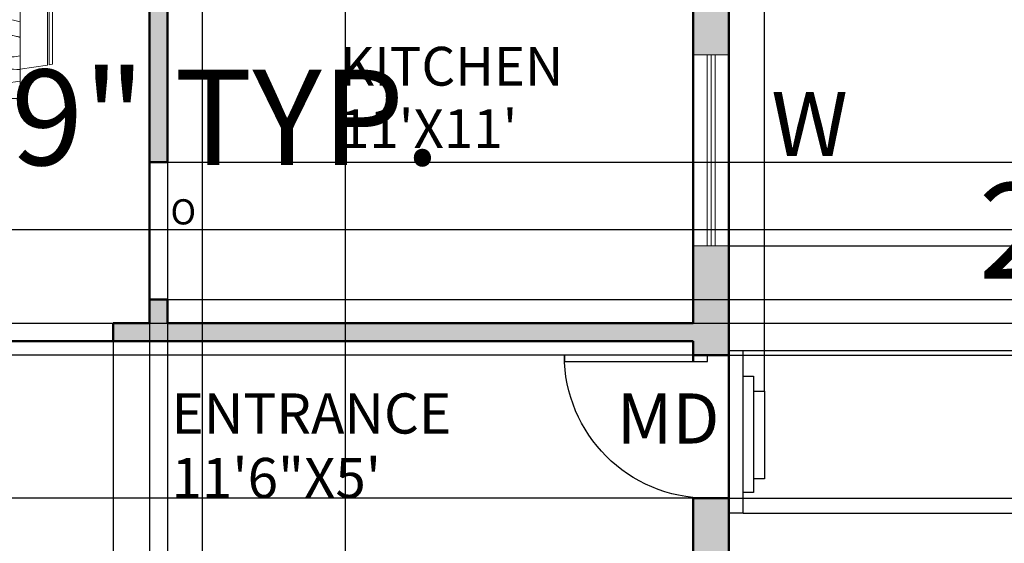
# Model space of a CAD drawing. Units: inches. Extents: x -166 to 1001, y 0 to 688.
# Tile 8 of 11: x 361 to 608, y 287 to 419. Entities that reach past the tile are written whole.
import ezdxf

# ---------------------------------------------------------------- set-up
doc = ezdxf.new("R2010")
doc.units = ezdxf.units.IN
doc.header["$MEASUREMENT"] = 0
for name, color, linetype, lineweight in [('A-ANNO-DIMS', 1, 'Continuous', 18), ('A-ANNO-TEXT', 2, 'Continuous', 25), ('A-AREA-IDEN', 2, 'Continuous', 25), ('A-DOOR', 6, 'Continuous', 25), ('A-FLOR-STRS', 7, 'Continuous', 25), ('A-GLAZ', 130, 'Continuous', 18), ('A-WALL-PATT', 5, 'Continuous', 13), ('FURNITURE', 11, 'Continuous', 18), ('WALLS', 250, 'Continuous', 50)]:
    doc.layers.add(name, color=color, linetype=linetype, lineweight=lineweight)
doc.styles.get("Standard").update_dxf_attribs({"font": 'arial.ttf'})
doc.dimstyles.get("Standard").update_dxf_attribs({"dimtxt": 24, "dimasz": 7, "dimexe": 0.18, "dimexo": 0.0625, "dimgap": 0.09, "dimtad": 0, "dimtih": 1, "dimtoh": 1, "dimdec": 0, "dimzin": 0, "dimdsep": 46, "dimlunit": 3, "dimtxsty": 'Standard', "dimcen": 0.09, "dimadec": 0, "dimazin": 0, "dimtfac": 1, "dimtdec": 0, "dimtofl": 0, "dimtmove": 0, "dimatfit": 3, "dimfxl": 1, "dimtolj": 1, "dimtzin": 0, "dimarcsym": 0})

# ---------------------------------------------------------------- blocks, each defined once
blk = doc.blocks.new('Dining Set - 36 x 72 in.')
for p, q in [((-22.2343, 26.00059), (-23.4847, 17.99762)), ((-22.2304, 26), (-5.7608, 26)), ((-22, 27.5), (-22.1562, 26.50042)), ((-5.8416, 26.5), (-22.1534, 26.5)), ((-22, 27.5), (-6, 27.5)), ((-5.8437, 26.49966), (-6, 27.5)), ((-4.5152, 17.99762), (-5.7655, 25.99926)), ((5.7657, 26.00059), (4.5153, 17.99762)), ((5.7696, 26), (22.2392, 26)), ((6, 27.5), (5.8438, 26.50042)), ((22.1584, 26.5), (5.8466, 26.5)), ((6, 27.5), (22, 27.5)), ((22.1563, 26.49966), (22, 27.5)), ((23.4848, 17.99762), (22.2345, 25.99926)), ((36, 18), (-36, 18)), ((-36, 18), (-36, -18)), ((36, -18), (36, 18)), ((-44.0006, 8.23428), (-35.9976, 9.48474)), ((44.0006, 8.23428), (35.9976, 9.48474)), ((-45.5, 8), (-44.5004, 8.15617)), ((-45.5, 8), (-45.5, -8)), ((-44.5, -8.15843), (-44.5, 8.15338)), ((-44, 8.23041), (-44, -8.23915)), ((44, 8.23041), (44, -8.23915)), ((44.5, -8.15843), (44.5, 8.15338)), ((45.5, 8), (44.5005, 8.15617)), ((45.5, 8), (45.5, -8)), ((-44.4997, -8.15631), (-45.5, -8)), ((-35.9976, -9.48476), (-43.9993, -8.2345)), ((35.9976, -9.48476), (43.9993, -8.2345)), ((44.4997, -8.15631), (45.5, -8)), ((-36, -18), (36, -18)), ((-22.2343, -26.0006), (-23.4847, -17.99762)), ((-4.5152, -17.99762), (-5.7655, -25.99928)), ((5.7657, -26.0006), (4.5153, -17.99762)), ((23.4848, -17.99762), (22.2345, -25.99928)), ((-22.2304, -26), (-5.7608, -26)), ((-22, -27.5), (-22.1562, -26.50044)), ((-5.8416, -26.5), (-22.1534, -26.5)), ((-22, -27.5), (-6, -27.5)), ((-5.8437, -26.49967), (-6, -27.5)), ((5.7696, -26), (22.2392, -26)), ((6, -27.5), (5.8438, -26.50044)), ((22.1584, -26.5), (5.8466, -26.5)), ((6, -27.5), (22, -27.5)), ((22.1563, -26.49967), (22, -27.5))]:
    blk.add_line(p, q)
for points in [[(-36, 15), (-31.1772, 14.97754), (-26.8079, 14.91406), (-22.8538, 14.81543), (-19.276, 14.6875), (-16.0362, 14.53613), (-13.0957, 14.36718), (-10.4159, 14.18652), (-7.9583, 14), (-5.6904, 13.81315), (-3.6035, 13.63021), (-1.6954, 13.45508), (0.0365, 13.29166), (1.5945, 13.14388), (2.9811, 13.01562), (4.1988, 12.9108), (5.25, 12.83333), (6.1393, 12.78613), (6.8802, 12.76823), (7.4883, 12.77767), (7.9792, 12.8125), (8.3685, 12.87077), (8.6719, 12.95052), (8.9049, 13.0498), (9.0833, 13.16666), (9.2205, 13.29899), (9.3216, 13.44401), (9.3895, 13.59879), (9.4271, 13.76041), (9.4373, 13.92594), (9.4232, 14.09245), (9.3875, 14.257), (9.3333, 14.41666), (9.2638, 14.56917), (9.1836, 14.71484), (9.0975, 14.85465), (9.0104, 14.98958), (8.9272, 15.1206), (8.8529, 15.2487), (8.7922, 15.37483), (8.75, 15.5), (8.7305, 15.62467), (8.7344, 15.74739), (8.7617, 15.86621), (8.8125, 15.97916), (8.8867, 16.08431), (8.9844, 16.17968), (9.1055, 16.26334), (9.25, 16.33333), (9.4189, 16.38802), (9.6172, 16.42708), (9.8506, 16.45052), (10.125, 16.45833), (10.4463, 16.45052), (10.8203, 16.42708), (11.2529, 16.38802), (11.75, 16.33333), (12.3184, 16.26318), (12.9694, 16.17838), (13.7151, 16.07991), (14.5677, 15.96875), (15.5395, 15.84586), (16.6426, 15.71224), (17.8893, 15.56884), (19.2917, 15.41666), (20.859, 15.25667), (22.5879, 15.08984), (24.4721, 14.91715), (26.5052, 14.73958), (28.6809, 14.5581), (30.9929, 14.3737), (33.4347, 14.18733), (36, 14)], [(-36, 10), (-28.9766, 10.14274), (-23.1725, 10.20442), (-18.4241, 10.19775), (-14.5677, 10.13541), (-11.4399, 10.03011), (-8.877, 9.89453), (-6.7154, 9.74137), (-4.7917, 9.58333), (-2.9698, 9.43082), (-1.2246, 9.28515), (0.4415, 9.14534), (2.026, 9.01041), (3.5266, 8.87939), (4.9408, 8.7513), (6.266, 8.62516), (7.5, 8.5), (8.6411, 8.37549), (9.6914, 8.2539), (10.6538, 8.13818), (11.5312, 8.03125), (12.3267, 7.93603), (13.043, 7.85547), (13.6831, 7.79248), (14.25, 7.75), (14.7471, 7.7303), (15.1797, 7.73307), (15.5537, 7.75732), (15.875, 7.80208), (16.1494, 7.86637), (16.3828, 7.94922), (16.5811, 8.04964), (16.75, 8.16666), (16.8944, 8.29915), (17.0143, 8.44531), (17.1089, 8.60319), (17.1771, 8.77083), (17.218, 8.94629), (17.2305, 9.1276), (17.2137, 9.31282), (17.1667, 9.5), (17.0895, 9.6875), (16.987, 9.875), (16.8649, 10.0625), (16.7292, 10.25), (16.5856, 10.4375), (16.4401, 10.625), (16.2985, 10.8125), (16.1667, 11), (16.05, 11.18733), (15.9518, 11.3737), (15.8752, 11.5581), (15.8229, 11.73958), (15.798, 11.91715), (15.8034, 12.08984), (15.842, 12.25667), (15.9167, 12.41666), (16.0295, 12.56836), (16.1784, 12.70833), (16.3605, 12.83268), (16.5729, 12.9375), (16.8127, 13.01888), (17.0768, 13.07291), (17.3625, 13.0957), (17.6667, 13.08333), (17.9894, 13.03312), (18.3418, 12.94726), (18.7382, 12.82918), (19.1927, 12.68229), (19.7195, 12.51001), (20.3327, 12.31575), (21.0465, 12.10294), (21.875, 11.875), (22.8357, 11.63354), (23.959, 11.37304), (25.2786, 11.08618), (26.8282, 10.76562), (28.6414, 10.40405), (30.752, 9.99414), (33.1936, 9.52856), (36, 9)], [(-36, 5.5), (-30.7157, 5.3348), (-26.069, 5.20963), (-21.9946, 5.11767), (-18.4271, 5.05208), (-15.3009, 5.00602), (-12.5508, 4.97265), (-10.1112, 4.94515), (-7.9167, 4.91666), (-5.909, 4.88167), (-4.0586, 4.83984), (-2.3429, 4.79215), (-0.7396, 4.73958), (0.7739, 4.6831), (2.22, 4.6237), (3.6213, 4.56233), (5, 4.5), (6.373, 4.43782), (7.7344, 4.3776), (9.0723, 4.32129), (10.375, 4.27083), (11.6309, 4.22819), (12.8281, 4.19531), (13.9551, 4.17415), (15, 4.16666), (15.954, 4.17448), (16.819, 4.19791), (17.6001, 4.23698), (18.3021, 4.29166), (18.9299, 4.36198), (19.4883, 4.44791), (19.9823, 4.54948), (20.4167, 4.66666), (20.7969, 4.79899), (21.1302, 4.94401), (21.4245, 5.09879), (21.6875, 5.26041), (21.9271, 5.42594), (22.1511, 5.59245), (22.3672, 5.757), (22.5834, 5.91666), (22.8065, 6.06868), (23.0404, 6.21093), (23.2879, 6.34147), (23.5521, 6.45833), (23.8358, 6.55957), (24.142, 6.64323), (24.4735, 6.70735), (24.8334, 6.75), (25.2235, 6.76969), (25.642, 6.76692), (26.0858, 6.74267), (26.5521, 6.69791), (27.0379, 6.63362), (27.5404, 6.55078), (28.0565, 6.45036), (28.5834, 6.33333), (29.1242, 6.19987), (29.7071, 6.04687), (30.3661, 5.87044), (31.1354, 5.66666), (32.0493, 5.43164), (33.142, 5.16146), (34.4475, 4.85221), (36, 4.5)], [(-36, -1), (-30.7915, -0.6591), (-26.0195, -0.38216), (-21.6519, -0.16284), (-17.6563, 0.00521), (-14.0005, 0.12833), (-10.6523, 0.21289), (-7.5796, 0.26522), (-4.75, 0.29166), (-2.134, 0.29793), (0.2878, 0.28711), (2.5317, 0.26163), (4.6146, 0.22396), (6.5529, 0.17651), (8.3633, 0.12174), (10.0623, 0.06209), (11.6667, 0), (13.1899, -0.06201), (14.6341, -0.1211), (15.9982, -0.17432), (17.2813, -0.21875), (18.4823, -0.25147), (19.6003, -0.26953), (20.6343, -0.27002), (21.5834, -0.25), (22.4481, -0.20768), (23.2357, -0.14584), (23.9549, -0.06836), (24.6146, 0.02083), (25.2235, 0.11784), (25.7904, 0.21875), (26.3241, 0.31966), (26.8334, 0.41666), (27.3265, 0.50618), (27.8099, 0.58593), (28.2894, 0.65397), (28.7709, 0.70833), (29.2601, 0.74707), (29.763, 0.76823), (30.2855, 0.76985), (30.8334, 0.75), (31.4088, 0.70784), (31.9994, 0.64713), (32.589, 0.57275), (33.1615, 0.48958), (33.7008, 0.4025), (34.1908, 0.3164), (34.6153, 0.23616), (34.9584, 0.16666), (35.2099, 0.11165), (35.3848, 0.07031), (35.504, 0.04069), (35.5886, 0.02083), (35.6594, 0.00879), (35.7377, 0.0026), (35.8442, 0.00032), (36, 0)], [(-36, -6.5), (-27.1843, -6.31267), (-20.084, -6.1263), (-14.469, -5.9419), (-10.1094, -5.76042), (-6.7752, -5.58285), (-4.2363, -5.41016), (-2.2629, -5.24333), (-0.625, -5.08334), (0.8708, -4.93099), (2.2715, -4.78646), (3.5872, -4.64974), (4.8281, -4.52084), (6.0046, -4.39974), (7.127, -4.28646), (8.2053, -4.18099), (9.25, -4.08334), (10.2705, -3.99382), (11.2734, -3.91407), (12.2647, -3.84603), (13.25, -3.79167), (14.2354, -3.75293), (15.2266, -3.73177), (16.2295, -3.73015), (17.25, -3.75), (18.2912, -3.79248), (19.3451, -3.85547), (20.4009, -3.93604), (21.4479, -4.03125), (22.4754, -4.13819), (23.4727, -4.25391), (24.4289, -4.37549), (25.3334, -4.5), (26.1785, -4.62492), (26.9694, -4.74935), (27.7145, -4.87281), (28.4219, -4.99479), (29.1, -5.11483), (29.7572, -5.23242), (30.4016, -5.34709), (31.0417, -5.45834), (31.6837, -5.56437), (32.3262, -5.65821), (32.9658, -5.73153), (33.599, -5.77604), (34.2224, -5.78345), (34.8327, -5.74545), (35.4264, -5.65373), (36, -5.5)], [(-36, -10), (-26.4022, -9.81299), (-18.4675, -9.62891), (-11.9839, -9.45069), (-6.7396, -9.28125), (-2.5226, -9.12354), (0.8789, -8.98047), (3.6769, -8.85498), (6.0833, -8.75), (8.2767, -8.66765), (10.3021, -8.60677), (12.1712, -8.56543), (13.8958, -8.54167), (15.4876, -8.53353), (16.9583, -8.53907), (18.3197, -8.55632), (19.5834, -8.58334), (20.7616, -8.61841), (21.8685, -8.66081), (22.9188, -8.71004), (23.9271, -8.76563), (24.9081, -8.82707), (25.8763, -8.89388), (26.8465, -8.96558), (27.8334, -9.04167), (28.8474, -9.12118), (29.8828, -9.20117), (30.93, -9.27824), (31.9792, -9.34896), (33.0205, -9.40991), (34.0443, -9.45768), (35.0407, -9.48885), (36, -9.5)], [(-36, -14.5), (-30.0881, -14.33513), (-25.0332, -14.21224), (-20.7312, -14.12647), (-17.0781, -14.07292), (-13.97, -14.04671), (-11.3027, -14.04297), (-8.9724, -14.05681), (-6.875, -14.08334), (-4.9224, -14.11833), (-3.0905, -14.16016), (-1.3709, -14.20785), (0.2448, -14.26042), (1.7647, -14.3169), (3.1973, -14.3763), (4.5507, -14.43767), (5.8333, -14.5), (7.0554, -14.5621), (8.235, -14.62175), (9.3922, -14.67652), (10.5469, -14.72396), (11.7192, -14.76164), (12.929, -14.78711), (14.1965, -14.79794), (15.5417, -14.79167), (16.9933, -14.76424), (18.6152, -14.70508), (20.4804, -14.60197), (22.6615, -14.44271), (25.2312, -14.21509), (28.2624, -13.9069), (31.8277, -13.50594), (36, -13)]]:
    blk.add_lwpolyline(points)
blk = doc.blocks.new('*U6')
for p, q in [((0, 0), (0, -6)), ((40, 0), (40, -6))]:
    blk.add_line(p, q)
blk.add_lwpolyline([(0, 0), (0, 40), (1.75, 40), (1.75, 0)], close=True)
blk.add_arc((0, 0), 40, 0, 90)
blk = doc.blocks.new('WIN-48IN')
for p, q in [((0, 4.5), (0, 9)), ((0, 9), (0, 0)), ((48, 9), (48, 0)), ((0, 5.5), (48, 5.5)), ((0, 4.5), (48, 4.5)), ((0, 3.5), (48, 3.5))]:
    blk.add_line(p, q)
blk = doc.blocks.new('*D21')
at = {"layer": 'A-ANNO-DIMS', "color": 0, "lineweight": -2, "transparency": 16777216}
for p, q in [((506.04, 225.45), (499.04, 225.45)), ((513.04, 226.95), (513.04, 225.27)), ((523.44, 226.95), (523.44, 225.27)), ((530.44, 225.45), (537.44, 225.45))]:
    blk.add_line(p, q, dxfattribs=at)
at = {"layer": 'A-ANNO-DIMS', "color": 0, "transparency": 16777216}
for points in [[(506.04, 226.62), (506.04, 224.29), (513.04, 225.45)], [(530.44, 226.62), (530.44, 224.29), (523.44, 225.45)]]:
    blk.add_solid(points, dxfattribs=at)
at = {"layer": 'Defpoints', "color": 0, "transparency": 16777216}
for p in [(513.04, 227.01), (523.44, 227.01), (523.44, 225.45)]:
    blk.add_point(p, dxfattribs=at)
at = {"layer": 'A-ANNO-DIMS', "color": 0, "transparency": 16777216, "insert": (775.99, 225.45), "char_height": 24, "attachment_point": 5}
blk.add_mtext('\\A1;BEDSIDE LAMP 0\'-10 1/2" TYP.', dxfattribs=at)
blk = doc.blocks.new('*D25')
at = {"layer": 'A-ANNO-DIMS', "color": 0, "lineweight": -2, "transparency": 16777216}
for p, q in [((218.36, 399.34), (218.36, 394.26)), ((251.4, 399.34), (251.4, 394.26)), ((225.36, 394.44), (244.4, 394.44)), ((251.4, 394.44), (258.4, 394.44))]:
    blk.add_line(p, q, dxfattribs=at)
at = {"layer": 'A-ANNO-DIMS', "color": 0, "transparency": 16777216}
for points in [[(225.36, 395.61), (225.36, 393.27), (218.36, 394.44)], [(244.4, 395.61), (244.4, 393.27), (251.4, 394.44)]]:
    blk.add_solid(points, dxfattribs=at)
at = {"layer": 'Defpoints', "color": 0, "transparency": 16777216}
for p in [(218.36, 399.4), (251.4, 399.4), (251.4, 394.44)]:
    blk.add_point(p, dxfattribs=at)
at = {"layer": 'A-ANNO-DIMS', "color": 0, "transparency": 16777216, "insert": (364.72, 394.44), "char_height": 24, "attachment_point": 5}
blk.add_mtext('\\A1;WC 2\'-9" TYP.', dxfattribs=at)
blk = doc.blocks.new('*D31')
at = {"layer": 'A-ANNO-DIMS', "color": 0, "lineweight": -2, "transparency": 16777216}
for p, q in [((484.56, 447.22), (484.56, 443.75)), ((506.92, 447.22), (506.92, 443.75)), ((491.56, 443.93), (499.92, 443.93)), ((506.92, 443.93), (513.92, 443.93))]:
    blk.add_line(p, q, dxfattribs=at)
at = {"layer": 'A-ANNO-DIMS', "color": 0, "transparency": 16777216}
for points in [[(491.56, 445.1), (491.56, 442.76), (484.56, 443.93)], [(499.92, 445.1), (499.92, 442.76), (506.92, 443.93)]]:
    blk.add_solid(points, dxfattribs=at)
at = {"layer": 'Defpoints', "color": 0, "transparency": 16777216}
for p in [(484.56, 447.28), (506.92, 447.28), (506.92, 443.93)]:
    blk.add_point(p, dxfattribs=at)
at = {"layer": 'A-ANNO-DIMS', "color": 0, "transparency": 16777216, "insert": (646.84, 443.93), "char_height": 24, "attachment_point": 5}
blk.add_mtext('\\A1;RANGE 1\'-10 1/2"', dxfattribs=at)
blk = doc.blocks.new('*D33')
at = {"layer": 'A-ANNO-DIMS', "color": 0, "lineweight": -2, "transparency": 16777216}
for p, q in [((291.16, 438.23), (291.16, 450.03)), ((369.04, 438.23), (369.04, 450.03)), ((298.16, 449.85), (362.04, 449.85)), ((369.04, 449.85), (376.04, 449.85))]:
    blk.add_line(p, q, dxfattribs=at)
at = {"layer": 'A-ANNO-DIMS', "color": 0, "transparency": 16777216}
for points in [[(298.16, 451.02), (298.16, 448.68), (291.16, 449.85)], [(362.04, 451.02), (362.04, 448.68), (369.04, 449.85)]]:
    blk.add_solid(points, dxfattribs=at)
at = {"layer": 'Defpoints', "color": 0, "transparency": 16777216}
for p in [(369.04, 449.85), (291.16, 438.17), (369.04, 438.17)]:
    blk.add_point(p, dxfattribs=at)
at = {"layer": 'A-ANNO-DIMS', "color": 0, "transparency": 16777216, "insert": (508.03, 449.85), "char_height": 24, "attachment_point": 5}
blk.add_mtext('\\A1;DINING SET 6\'-6"', dxfattribs=at)
blk = doc.blocks.new('*D46')
at = {"layer": 'A-ANNO-DIMS', "color": 0, "lineweight": -2, "transparency": 16777216}
for p, q in [((261.38, 474.68), (261.38, 35.41)), ((298.66, 474.68), (298.66, 35.41)), ((268.38, 35.59), (291.66, 35.59)), ((298.66, 35.59), (305.66, 35.59))]:
    blk.add_line(p, q, dxfattribs=at)
at = {"layer": 'A-ANNO-DIMS', "color": 0, "transparency": 16777216}
for points in [[(268.38, 36.76), (268.38, 34.42), (261.38, 35.59)], [(291.66, 36.76), (291.66, 34.42), (298.66, 35.59)]]:
    blk.add_solid(points, dxfattribs=at)
at = {"layer": 'Defpoints', "color": 0, "transparency": 16777216}
for p in [(261.38, 474.74), (298.66, 474.74), (298.66, 35.59)]:
    blk.add_point(p, dxfattribs=at)
at = {"layer": 'A-ANNO-DIMS', "color": 0, "transparency": 16777216, "insert": (365.61, 35.59), "char_height": 24, "attachment_point": 5}
blk.add_mtext('\\A1;3\'-1 1/2"', dxfattribs=at)
blk = doc.blocks.new('*D52')
at = {"layer": 'A-ANNO-DIMS', "color": 0, "lineweight": -2, "transparency": 16777216}
for p, q in [((675.03, 366.29), (675.03, 373.29)), ((675.03, 373.29), (682.03, 373.29)), ((24.44, 366.29), (675.21, 366.29)), ((675.03, 349.74), (675.03, 359.29)), ((24.44, 342.74), (675.21, 342.74))]:
    blk.add_line(p, q, dxfattribs=at)
at = {"layer": 'A-ANNO-DIMS', "color": 0, "transparency": 16777216}
for points in [[(673.87, 359.29), (676.2, 359.29), (675.03, 366.29)], [(673.87, 349.74), (676.2, 349.74), (675.03, 342.74)]]:
    blk.add_solid(points, dxfattribs=at)
at = {"layer": 'Defpoints', "color": 0, "transparency": 16777216}
for p in [(24.38, 366.29), (675.03, 366.29), (24.38, 342.74)]:
    blk.add_point(p, dxfattribs=at)
at = {"layer": 'A-ANNO-DIMS', "color": 0, "transparency": 16777216, "insert": (750.18, 373.29), "char_height": 24, "attachment_point": 5}
blk.add_mtext('\\A1;1\'-11 1/2"', dxfattribs=at)
blk = doc.blocks.new('*D54')
at = {"layer": 'A-ANNO-DIMS', "color": 0, "lineweight": -2, "transparency": 16777216}
for p, q in [((538.94, 298.79), (675.21, 298.79)), ((675.03, 291.79), (675.03, 272.71)), ((675.03, 228.94), (675.03, 248.02)), ((538.94, 221.94), (675.21, 221.94))]:
    blk.add_line(p, q, dxfattribs=at)
at = {"layer": 'A-ANNO-DIMS', "color": 0, "transparency": 16777216}
for points in [[(673.87, 291.79), (676.2, 291.79), (675.03, 298.79)], [(673.87, 228.94), (676.2, 228.94), (675.03, 221.94)]]:
    blk.add_solid(points, dxfattribs=at)
at = {"layer": 'Defpoints', "color": 0, "transparency": 16777216}
for p in [(538.88, 298.79), (675.03, 298.79), (538.88, 221.94)]:
    blk.add_point(p, dxfattribs=at)
at = {"layer": 'A-ANNO-DIMS', "color": 0, "transparency": 16777216, "insert": (675.03, 260.36), "char_height": 24, "attachment_point": 5}
blk.add_mtext('\\A1;6\'-5"', dxfattribs=at)
blk = doc.blocks.new('*D55')
at = {"layer": 'A-ANNO-DIMS', "color": 0, "lineweight": -2, "transparency": 16777216}
for p, q in [((-120.77, 341.73), (-120.77, 348.73)), ((529.82, 334.73), (-120.95, 334.73)), ((529.82, 298.79), (-120.95, 298.79)), ((-120.77, 291.79), (-120.77, 284.79))]:
    blk.add_line(p, q, dxfattribs=at)
at = {"layer": 'A-ANNO-DIMS', "color": 0, "transparency": 16777216}
for points in [[(-121.93, 341.73), (-119.6, 341.73), (-120.77, 334.73)], [(-121.93, 291.79), (-119.6, 291.79), (-120.77, 298.79)]]:
    blk.add_solid(points, dxfattribs=at)
at = {"layer": 'Defpoints', "color": 0, "transparency": 16777216}
for p in [(-120.77, 334.73), (529.88, 334.73), (529.88, 298.79)]:
    blk.add_point(p, dxfattribs=at)
at = {"layer": 'A-ANNO-DIMS', "color": 0, "transparency": 16777216, "insert": (-120.77, 316.76), "char_height": 24, "attachment_point": 5}
blk.add_mtext('\\A1;3\'-0"', dxfattribs=at)
blk = doc.blocks.new('*D56')
at = {"layer": 'A-ANNO-DIMS', "color": 0, "lineweight": -2, "transparency": 16777216}
for p, q in [((675.03, 369.18), (675.03, 376.18)), ((538.94, 362.18), (675.21, 362.18)), ((538.94, 334.73), (675.21, 334.73)), ((675.03, 327.73), (675.03, 320.73))]:
    blk.add_line(p, q, dxfattribs=at)
at = {"layer": 'A-ANNO-DIMS', "color": 0, "transparency": 16777216}
for points in [[(673.87, 369.18), (676.2, 369.18), (675.03, 362.18)], [(673.87, 327.73), (676.2, 327.73), (675.03, 334.73)]]:
    blk.add_solid(points, dxfattribs=at)
at = {"layer": 'Defpoints', "color": 0, "transparency": 16777216}
for p in [(538.88, 362.18), (675.03, 362.18), (538.88, 334.73)]:
    blk.add_point(p, dxfattribs=at)
at = {"layer": 'A-ANNO-DIMS', "color": 0, "transparency": 16777216, "insert": (675.03, 348.46), "char_height": 24, "attachment_point": 5}
blk.add_mtext('\\A1;2\'-3 1/2"', dxfattribs=at)
blk = doc.blocks.new('*D57')
at = {"layer": 'A-ANNO-DIMS', "color": 0, "lineweight": -2, "transparency": 16777216}
for p, q in [((531.88, 592.89), (524.88, 592.89)), ((538.88, 335.97), (538.88, 593.07)), ((547.76, 325.77), (547.76, 593.07)), ((554.76, 592.89), (561.76, 592.89))]:
    blk.add_line(p, q, dxfattribs=at)
at = {"layer": 'A-ANNO-DIMS', "color": 0, "transparency": 16777216}
for points in [[(531.88, 594.06), (531.88, 591.72), (538.88, 592.89)], [(554.76, 594.06), (554.76, 591.72), (547.76, 592.89)]]:
    blk.add_solid(points, dxfattribs=at)
at = {"layer": 'Defpoints', "color": 0, "transparency": 16777216}
for p in [(547.76, 592.89), (538.88, 335.91), (547.76, 325.71)]:
    blk.add_point(p, dxfattribs=at)
at = {"layer": 'A-ANNO-DIMS', "color": 0, "transparency": 16777216, "insert": (593.75, 592.89), "char_height": 24, "attachment_point": 5}
blk.add_mtext('\\A1;0\'-9"', dxfattribs=at)
blk = doc.blocks.new('*D58')
at = {"layer": 'A-ANNO-DIMS', "color": 0, "lineweight": -2, "transparency": 16777216}
for p, q in [((542.41, 335.91), (675.21, 335.91)), ((675.03, 328.91), (675.03, 327.8)), ((675.03, 301.99), (675.03, 303.1)), ((542.41, 294.99), (675.21, 294.99))]:
    blk.add_line(p, q, dxfattribs=at)
at = {"layer": 'A-ANNO-DIMS', "color": 0, "transparency": 16777216}
for points in [[(673.87, 328.91), (676.2, 328.91), (675.03, 335.91)], [(673.87, 301.99), (676.2, 301.99), (675.03, 294.99)]]:
    blk.add_solid(points, dxfattribs=at)
at = {"layer": 'Defpoints', "color": 0, "transparency": 16777216}
for p in [(542.35, 335.91), (542.35, 294.99), (675.03, 294.99)]:
    blk.add_point(p, dxfattribs=at)
at = {"layer": 'A-ANNO-DIMS', "color": 0, "transparency": 16777216, "insert": (675.03, 315.45), "char_height": 24, "attachment_point": 5}
blk.add_mtext('\\A1;3\'-5"', dxfattribs=at)
blk = doc.blocks.new('*D62')
at = {"layer": 'A-ANNO-DIMS', "color": 0, "lineweight": -2, "transparency": 16777216}
for p, q in [((201.55, 342.8), (201.55, 593.07)), ((208.55, 592.89), (249.88, 592.89)), ((256.88, 342.8), (256.88, 593.07)), ((256.88, 592.89), (263.88, 592.89))]:
    blk.add_line(p, q, dxfattribs=at)
at = {"layer": 'A-ANNO-DIMS', "color": 0, "transparency": 16777216}
for points in [[(208.55, 594.06), (208.55, 591.72), (201.55, 592.89)], [(249.88, 594.06), (249.88, 591.72), (256.88, 592.89)]]:
    blk.add_solid(points, dxfattribs=at)
at = {"layer": 'Defpoints', "color": 0, "transparency": 16777216}
for p in [(256.88, 592.89), (201.55, 342.74), (256.88, 342.74)]:
    blk.add_point(p, dxfattribs=at)
at = {"layer": 'A-ANNO-DIMS', "color": 0, "transparency": 16777216, "insert": (324.32, 592.89), "char_height": 24, "attachment_point": 5}
blk.add_mtext('\\A1;4\'-7 1/2"', dxfattribs=at)
blk = doc.blocks.new('*D63')
at = {"layer": 'A-ANNO-DIMS', "color": 0, "lineweight": -2, "transparency": 16777216}
for p, q in [((274.49, 338.18), (274.49, 35.41)), ((384.24, 338.18), (384.24, 35.41)), ((281.49, 35.59), (377.24, 35.59)), ((384.24, 35.59), (391.24, 35.59))]:
    blk.add_line(p, q, dxfattribs=at)
at = {"layer": 'A-ANNO-DIMS', "color": 0, "transparency": 16777216}
for points in [[(281.49, 36.76), (281.49, 34.42), (274.49, 35.59)], [(377.24, 36.76), (377.24, 34.42), (384.24, 35.59)]]:
    blk.add_solid(points, dxfattribs=at)
at = {"layer": 'Defpoints', "color": 0, "transparency": 16777216}
for p in [(274.49, 338.24), (384.24, 338.24), (384.24, 35.59)]:
    blk.add_point(p, dxfattribs=at)
at = {"layer": 'A-ANNO-DIMS', "color": 0, "transparency": 16777216, "insert": (451.19, 35.59), "char_height": 24, "attachment_point": 5}
blk.add_mtext('\\A1;9\'-1 1/2"', dxfattribs=at)
blk = doc.blocks.new('*D65')
at = {"layer": 'A-ANNO-DIMS', "color": 0, "lineweight": -2, "transparency": 16777216}
for p, q in [((675.03, 390.21), (675.03, 397.21)), ((397.94, 383.21), (675.21, 383.21)), ((397.94, 348.69), (675.21, 348.69)), ((675.03, 341.69), (675.03, 334.69))]:
    blk.add_line(p, q, dxfattribs=at)
at = {"layer": 'A-ANNO-DIMS', "color": 0, "transparency": 16777216}
for points in [[(673.87, 390.21), (676.2, 390.21), (675.03, 383.21)], [(673.87, 341.69), (676.2, 341.69), (675.03, 348.69)]]:
    blk.add_solid(points, dxfattribs=at)
at = {"layer": 'Defpoints', "color": 0, "transparency": 16777216}
for p in [(397.88, 383.21), (675.03, 383.21), (397.88, 348.69)]:
    blk.add_point(p, dxfattribs=at)
at = {"layer": 'A-ANNO-DIMS', "color": 0, "transparency": 16777216, "insert": (675.03, 365.95), "char_height": 24, "attachment_point": 5}
blk.add_mtext('\\A1;2\'-10 1/2"', dxfattribs=at)
blk = doc.blocks.new('*D66')
at = {"layer": 'A-ANNO-DIMS', "color": 0, "lineweight": -2, "transparency": 16777216}
for p, q in [((675.03, 355.69), (675.03, 362.69)), ((675.03, 362.69), (682.03, 362.69)), ((397.94, 348.69), (675.21, 348.69)), ((397.94, 342.74), (675.21, 342.74)), ((675.03, 335.74), (675.03, 328.74))]:
    blk.add_line(p, q, dxfattribs=at)
at = {"layer": 'A-ANNO-DIMS', "color": 0, "transparency": 16777216}
for points in [[(673.87, 355.69), (676.2, 355.69), (675.03, 348.69)], [(673.87, 335.74), (676.2, 335.74), (675.03, 342.74)]]:
    blk.add_solid(points, dxfattribs=at)
at = {"layer": 'Defpoints', "color": 0, "transparency": 16777216}
for p in [(397.88, 348.69), (675.03, 348.69), (397.88, 342.74)]:
    blk.add_point(p, dxfattribs=at)
at = {"layer": 'A-ANNO-DIMS', "color": 0, "transparency": 16777216, "insert": (714.02, 362.69), "char_height": 24, "attachment_point": 5}
blk.add_mtext('\\A1;0\'-6"', dxfattribs=at)
blk = doc.blocks.new('*D71')
at = {"layer": 'A-ANNO-DIMS', "color": 0, "lineweight": -2, "transparency": 16777216}
for p, q in [((406.66, 278.3), (406.66, 593.07)), ((413.66, 592.89), (435.61, 592.89)), ((442.61, 278.3), (442.61, 593.07)), ((442.61, 592.89), (449.61, 592.89))]:
    blk.add_line(p, q, dxfattribs=at)
at = {"layer": 'A-ANNO-DIMS', "color": 0, "transparency": 16777216}
for points in [[(413.66, 594.06), (413.66, 591.72), (406.66, 592.89)], [(435.61, 594.06), (435.61, 591.72), (442.61, 592.89)]]:
    blk.add_solid(points, dxfattribs=at)
at = {"layer": 'Defpoints', "color": 0, "transparency": 16777216}
for p in [(442.61, 592.89), (406.66, 278.24), (442.61, 278.24)]:
    blk.add_point(p, dxfattribs=at)
at = {"layer": 'A-ANNO-DIMS', "color": 0, "transparency": 16777216, "insert": (481.59, 592.89), "char_height": 24, "attachment_point": 5}
blk.add_mtext('\\A1;3\'-0"', dxfattribs=at)
blk = doc.blocks.new('*D80')
at = {"layer": 'A-ANNO-DIMS', "color": 0, "lineweight": -2, "transparency": 16777216}
for p, q in [((393.38, 383.15), (393.38, 35.41)), ((397.88, 383.15), (397.88, 35.41)), ((386.38, 35.59), (379.38, 35.59)), ((404.88, 35.59), (411.88, 35.59))]:
    blk.add_line(p, q, dxfattribs=at)
at = {"layer": 'A-ANNO-DIMS', "color": 0, "transparency": 16777216}
for points in [[(386.38, 36.76), (386.38, 34.42), (393.38, 35.59)], [(404.88, 36.76), (404.88, 34.42), (397.88, 35.59)]]:
    blk.add_solid(points, dxfattribs=at)
at = {"layer": 'Defpoints', "color": 0, "transparency": 16777216}
for p in [(393.38, 383.21), (397.88, 383.21), (397.88, 35.59)]:
    blk.add_point(p, dxfattribs=at)
at = {"layer": 'A-ANNO-DIMS', "color": 0, "transparency": 16777216, "insert": (471.83, 35.59), "char_height": 24, "attachment_point": 5}
blk.add_mtext('\\A1;0\'-4 1/2"', dxfattribs=at)

msp = doc.modelspace()

# ---------------------------------------------------------------- hatches: boundary and pattern name
at = {"layer": 'A-WALL-PATT'}
h = msp.add_hatch(color=256, dxfattribs=at)
h.dxf.hatch_style = 1
h.paths.add_polyline_path([(96.05, 483.74), (15.38, 483.74), (15.38, 414.29), (24.38, 414.29), (24.38, 474.74), (96.05, 474.74)])
h.paths.add_polyline_path([(175.47, 483.74), (144.05, 483.74), (144.05, 474.74), (156.38, 474.74), (175.47, 474.74)])
h.paths.add_polyline_path([(298.66, 483.74), (199.47, 483.74), (199.47, 474.74), (256.88, 474.74), (298.66, 474.74)])
h.paths.add_polyline_path([(430.46, 483.74), (346.66, 483.74), (346.66, 474.74), (393.38, 474.74), (430.46, 474.74)])
h.paths.add_polyline_path([(261.38, 474.74), (256.88, 474.74), (256.88, 342.74), (201.55, 342.74), (201.55, 338.24), (274.49, 338.24), (274.49, 342.74), (261.38, 342.74)])
h.paths.add_polyline_path([(160.88, 474.74), (156.38, 474.74), (156.38, 342.74), (146.03, 342.74), (146.03, 338.24), (171.55, 338.24), (171.55, 342.74), (160.88, 342.74)])
h.paths.add_polyline_path([(397.88, 474.74), (393.38, 474.74), (393.38, 383.21), (397.88, 383.21)])
h.paths.add_polyline_path([(538.88, 362.18), (529.88, 362.18), (529.88, 342.74), (397.88, 342.74), (397.88, 348.69), (393.38, 348.69), (393.38, 342.74), (384.24, 342.74), (384.24, 338.24), (529.88, 338.24), (529.88, 334.73), (538.88, 334.73)])
h.paths.add_polyline_path([(538.88, 483.74), (478.46, 483.74), (478.46, 474.74), (529.88, 474.74), (529.88, 410.18), (538.88, 410.18)])
h.paths.add_polyline_path([(538.88, 298.79), (529.88, 298.79), (529.88, 278.24), (442.61, 278.24), (442.61, 273.74), (529.88, 273.74), (529.88, 221.94), (538.88, 221.94)])
h.paths.add_polyline_path([(538.88, 173.94), (529.88, 173.94), (529.88, 153.74), (393.38, 153.74), (382.23, 153.74), (382.23, 144.74), (538.88, 144.74)])
h.paths.add_polyline_path([(397.88, 164.32), (393.38, 164.32), (393.38, 153.74), (397.88, 153.74)], flags=17)
h.paths.add_polyline_path([(397.88, 273.74), (406.66, 273.74), (406.66, 278.24), (393.38, 278.24), (393.38, 273.74), (393.38, 230.24), (316.88, 230.24), (316.88, 153.74), (321.38, 153.74), (321.38, 225.74), (393.38, 225.74), (393.38, 194.32), (397.88, 194.32)])
h.paths.add_polyline_path([(358.23, 153.74), (316.88, 153.74), (284.58, 153.74), (284.58, 144.74), (358.23, 144.74)])
h.paths.add_polyline_path([(224.58, 153.74), (156.38, 153.74), (149.31, 153.74), (149.31, 144.74), (224.58, 144.74)])
h.paths.add_polyline_path([(101.31, 153.74), (24.38, 153.74), (24.38, 168.41), (15.38, 168.41), (15.38, 144.74), (101.31, 144.74)])
h.paths.add_polyline_path([(160.88, 273.74), (160.88, 278.24), (147.87, 278.24), (147.87, 273.74), (156.38, 273.74), (156.38, 153.74), (160.88, 153.74)])
h.paths.add_polyline_path([(111.92, 278.24), (100.88, 278.24), (100.88, 338.24), (110.03, 338.24), (110.03, 342.74), (24.38, 342.74), (24.38, 366.29), (15.38, 366.29), (15.38, 216.41), (24.38, 216.41), (24.38, 273.74), (44.93, 273.74), (44.93, 278.24), (24.38, 278.24), (24.38, 338.24), (96.38, 338.24), (96.38, 278.24), (74.93, 278.24), (74.93, 273.74), (111.92, 273.74)])

# ---------------------------------------------------------------- linework, layer by layer
at = {"layer": 'A-FLOR-STRS'}
for p, q in [((538.88, 335.91), (542.35, 335.91)), ((542.35, 335.91), (542.35, 294.99)), ((542.35, 329.47), (545, 329.47)), ((545, 329.47), (545, 300.19)), ((545, 325.71), (547.76, 325.71)), ((547.76, 325.71), (547.76, 303.63)), ((547.76, 303.63), (545, 303.63)), ((545, 300.19), (542.35, 300.19)), ((542.35, 294.99), (538.88, 294.99))]:
    msp.add_line(p, q, dxfattribs=at)
at = {"layer": 'WALLS'}
for p, q in [((538.88, 144.74), (538.88, 483.74)), ((393.38, 342.74), (393.38, 474.74)), ((397.88, 383.21), (397.88, 474.74)), ((529.88, 342.74), (529.88, 474.74)), ((393.38, 383.21), (397.88, 383.21)), ((393.38, 348.69), (397.88, 348.69)), ((397.88, 342.74), (397.88, 348.69)), ((384.24, 342.74), (384.24, 338.24)), ((384.24, 342.74), (393.38, 342.74)), ((397.88, 342.74), (529.88, 342.74)), ((201.55, 338.24), (529.88, 338.24)), ((529.88, 333.16), (529.88, 338.24)), ((529.88, 334.73), (538.88, 334.73)), ((529.88, 278.24), (529.88, 298.97)), ((538.88, 298.79), (529.88, 298.79))]:
    msp.add_line(p, q, dxfattribs=at)

# ---------------------------------------------------------------- block references
at = {"layer": 'A-DOOR', "xscale": -0.8986699555462259, "yscale": 0.8986699555462259, "zscale": 0.8986699555462259, "rotation": 90}
msp.add_blockref('*U6', (533.49, 334.73), dxfattribs=at)
at = {"layer": 'A-GLAZ', "rotation": 89.9999999999992}
msp.add_blockref('WIN-48IN', (538.88, 362.18), dxfattribs=at)
at = {"layer": 'FURNITURE', "xscale": 0.8558305474851317, "yscale": 0.8558305474851317, "zscale": 0.8558305474851317}
msp.add_blockref('Dining Set - 36 x 72 in.', (330.1, 414.63), dxfattribs=at)

# ---------------------------------------------------------------- texts
at = {"layer": 'A-ANNO-TEXT'}
for s, height, p in [('W ', 16.096, (549.48, 384.75)), ('MD', 12.597, (510.72, 312.51))]:
    msp.add_text(s, height=height, dxfattribs=at).set_placement(p)
msp.add_text('O', height=6.33, rotation=180, dxfattribs=at).set_placement((405.07, 373.88))
at = {"layer": 'A-AREA-IDEN'}
for s, height, p in [('KITCHEN ', 9.752, (441.2, 402.41)), ("11'X11'", 9.752, (441.2, 386.74)), ('ENTRANCE', 10.084, (398.92, 315.02)), ('11\'6"X5\'', 10.084, (398.92, 298.82))]:
    msp.add_text(s, height=height, dxfattribs=at).set_placement(p)

# ---------------------------------------------------------------- dimensions: what is measured, and where the dimension line sits
at = {"layer": 'A-ANNO-DIMS'}
for base, p1, p2, picture, middle in [((256.88, 592.89), (201.55, 342.74), (256.88, 342.74), '*D62', (324.32, 592.89)), ((442.6082, 592.8909), (406.6614, 278.2409), (442.6082, 278.2409), '*D71', (481.589, 592.8909)), ((547.76, 592.89), (538.88, 335.91), (547.76, 325.71), '*D57', (593.75, 592.89)), ((298.66, 35.59), (261.38, 474.74), (298.66, 474.74), '*D46', (365.61, 35.59)), ((397.88, 35.59), (393.38, 383.21), (397.88, 383.21), '*D80', (471.83, 35.59)), ((384.2404, 35.5909), (274.4932, 338.2409), (384.2404, 338.2409), '*D63', (451.1912, 35.5909))]:
    dim = msp.add_linear_dim(base=base, p1=p1, p2=p2, dimstyle='Standard', override={"dimdec": 1, "dimlfac": 1, "dimrnd": 0, "dimzin": 1, "dimdsep": 46, "dimlunit": 4, "dimfrac": 2}, dxfattribs=at)
    dim.commit()
    dim.dimension.update_dxf_attribs({"geometry": picture, "text_midpoint": middle})
for base, p1, p2, text, picture, middle in [((369.04, 449.85), (291.16, 438.17), (369.04, 438.17), 'DINING SET <>', '*D33', (508.03, 449.85)), ((506.92, 443.93), (484.56, 447.28), (506.92, 447.28), 'RANGE <>', '*D31', (646.84, 443.93)), ((251.4, 394.44), (218.36, 399.4), (251.4, 399.4), 'WC <> TYP.', '*D25', (364.72, 394.44)), ((523.44, 225.45), (513.04, 227.01), (523.44, 227.01), 'BEDSIDE LAMP <> TYP.', '*D21', (775.99, 225.45))]:
    dim = msp.add_linear_dim(base=base, p1=p1, p2=p2, text=text, dimstyle='Standard', override={"dimdec": 1, "dimlfac": 1, "dimrnd": 0, "dimzin": 1, "dimdsep": 46, "dimlunit": 4, "dimfrac": 2}, dxfattribs=at)
    dim.commit()
    dim.dimension.update_dxf_attribs({"geometry": picture, "text_midpoint": middle})
for base, p1, p2, picture, middle in [((675.0325, 366.2884), (24.3825, 342.7409), (24.3825, 366.2884), '*D52', (750.177, 373.2884)), ((675.03, 383.21), (397.88, 348.69), (397.88, 383.21), '*D65', (675.03, 365.95)), ((675.0325, 362.1777), (538.8825, 334.734), (538.8825, 362.1777), '*D56', (675.0325, 348.4559)), ((675.0325, 348.6892), (397.8825, 342.7409), (397.8825, 348.6892), '*D66', (714.0215, 362.6892)), ((-120.77, 334.73), (529.88, 298.79), (529.88, 334.73), '*D55', (-120.77, 316.76)), ((675.03, 294.99), (542.35, 335.91), (542.35, 294.99), '*D58', (675.03, 315.45)), ((675.0325, 298.7872), (538.8825, 221.9421), (538.8825, 298.7872), '*D54', (675.0325, 260.3646))]:
    dim = msp.add_linear_dim(base=base, p1=p1, p2=p2, angle=90, dimstyle='Standard', override={"dimdec": 1, "dimlfac": 1, "dimrnd": 0, "dimzin": 1, "dimdsep": 46, "dimlunit": 4, "dimfrac": 2}, dxfattribs=at)
    dim.commit()
    dim.dimension.update_dxf_attribs({"geometry": picture, "text_midpoint": middle})

doc.saveas('drawing.dxf')
